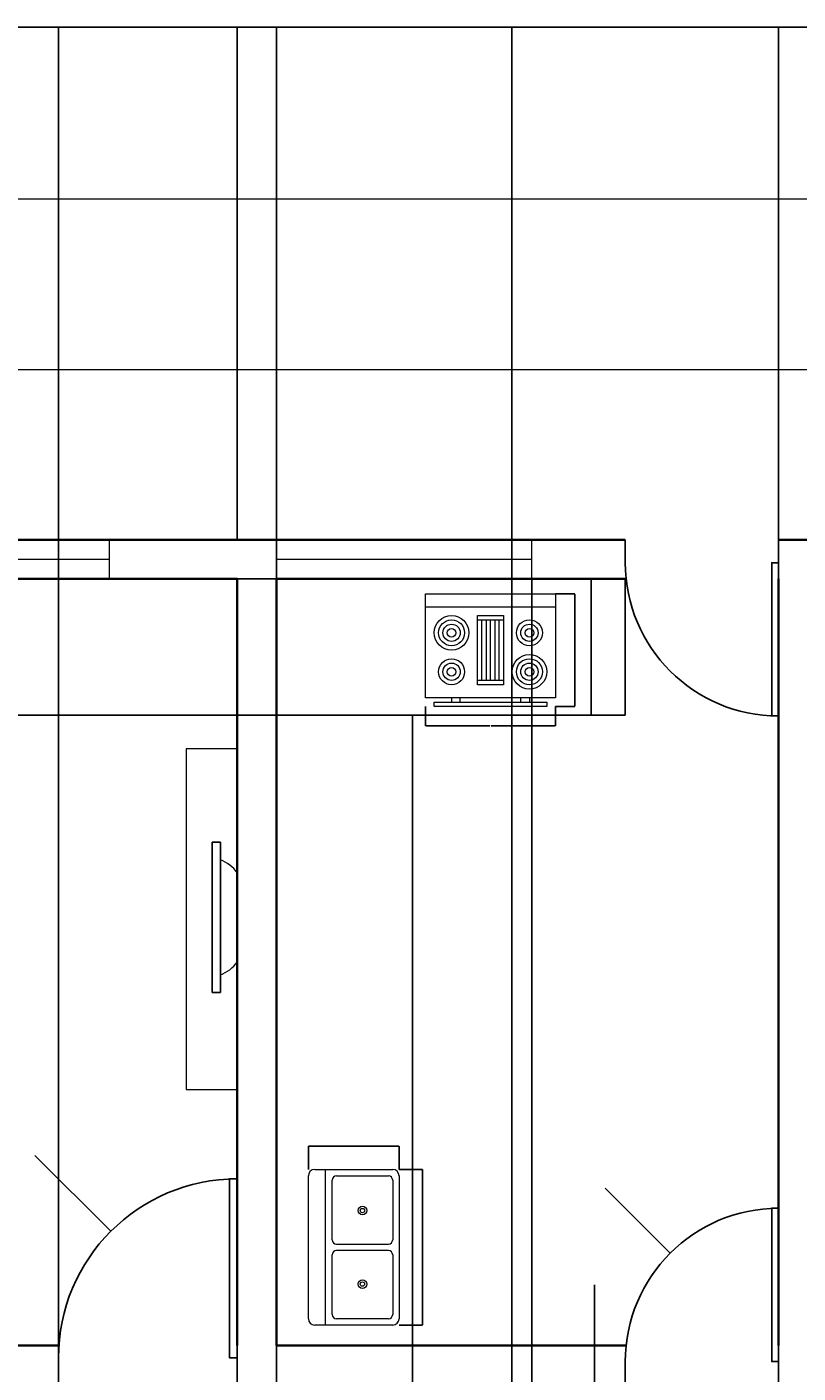
# Model space of a CAD drawing. Units: millimetres. Extents: x -8052 to 19968, y -37825 to -17505.
# Tile 7 of 10: x -516 to 4015, y -25407 to -17505. Entities that reach past the tile are written whole.
import ezdxf

# ---------------------------------------------------------------- set-up
doc = ezdxf.new("R2010")
doc.units = ezdxf.units.MM
doc.header["$MEASUREMENT"] = 0
for name, color, linetype, lineweight in [('A-ANNO-DIMS', 2, 'Continuous', 18), ('A-DOOR', 3, 'Continuous', 25), ('A-EQPM', 8, 'Continuous', 18), ('A-FLOR', 8, 'Continuous', 18), ('A-FLOR-CASE', 9, 'Continuous', 25), ('A-FLOR-FIXT', 9, 'Continuous', 18), ('A-GLAZ', 4, 'Continuous', 18), ('A-WALL', 7, 'Continuous', 35)]:
    doc.layers.add(name, color=color, linetype=linetype, lineweight=lineweight)
doc.styles.get("Standard").update_dxf_attribs({"font": 'arial.ttf'})
doc.dimstyles.get("Standard").update_dxf_attribs({"dimtxt": 1.054, "dimasz": 1.055, "dimexe": 0.18, "dimexo": 0.0625, "dimgap": 0.09, "dimtad": 0, "dimtih": 1, "dimtoh": 1, "dimdec": 4, "dimzin": 0, "dimdsep": 46, "dimtxsty": 'Standard', "dimcen": 0.09, "dimadec": 0, "dimazin": 0, "dimtfac": 1, "dimtdec": 4, "dimtofl": 0, "dimtmove": 0, "dimatfit": 3, "dimfxl": 1, "dimtolj": 1, "dimtzin": 0, "dimarcsym": 0})

# ---------------------------------------------------------------- blocks, each defined once
blk = doc.blocks.new('*U10')
for p, q in [((0, 0), (0, -6)), ((40, 0), (40, -6))]:
    blk.add_line(p, q)
blk.add_lwpolyline([(0, 0), (0, 40), (1.75, 40), (1.75, 0)], close=True)
blk.add_arc((0, 0), 40, 0, 90)
blk = doc.blocks.new('Range-Oven - 30 in top')
for p, q in [((0, -3), (30, -3)), ((12, -6), (18, -6)), ((13, -20), (13, -6)), ((14, -6), (14, -20)), ((15, -20), (15, -6)), ((16, -6), (16, -20)), ((17, -20), (17, -6)), ((18, -20), (12, -20)), ((6, -24), (6, -25)), ((8, -25), (8, -24)), ((22, -25), (22, -24)), ((24, -24), (24, -25))]:
    blk.add_line(p, q)
for points in [[(0, -24), (0, 0), (30, 0), (30, -24)], [(12, -21), (12, -5), (18, -5), (18, -21)], [(2, -26), (2, -25), (28, -25), (28, -26)]]:
    blk.add_lwpolyline(points, close=True)
for centre, radius in [((6, -9), 4), ((6, -9), 3), ((24, -9), 3), ((6, -9), 2), ((6, -9), 1), ((24, -9), 2), ((24, -9), 1), ((6, -18), 3), ((24, -18), 4), ((24, -18), 3), ((6, -18), 2), ((6, -18), 1), ((24, -18), 2), ((24, -18), 1)]:
    blk.add_circle(centre, radius)
blk = doc.blocks.new('Sink-double - 36 in top')
for p, q in [((-18, -4), (18, -4)), ((-0.75, -18.5), (-0.75, -6.5)), ((0.75, -6.5), (0.75, -18.5))]:
    blk.add_line(p, q)
for points in [[(-16.5, 0), (16.5, 0)], [(-18, -19.5), (-18, -1.5)], [(18, -1.5), (18, -19.5)], [(-15.5, -5.5), (-1.75, -5.5)], [(1.75, -5.5), (15.5, -5.5)], [(-16.5, -18.5), (-16.5, -6.5)], [(16.5, -6.5), (16.5, -18.5)], [(16.5, -21), (-16.5, -21)], [(-1.75, -19.5), (-15.5, -19.5)], [(15.5, -19.5), (1.75, -19.5)]]:
    blk.add_lwpolyline(points)
for centre, radius in [((-8.5, -12.5), 1), ((-8.5, -12.5), 0.5), ((8.5, -12.5), 1), ((8.5, -12.5), 0.5)]:
    blk.add_circle(centre, radius)
for centre, radius, start, end in [((-16.5, -1.5), 1.5, 90, 180), ((16.5, -1.5), 1.5, 0, 90), ((-15.5, -6.5), 1, 90, 180), ((-1.75, -6.5), 1, 0, 90), ((1.75, -6.5), 1, 90, 180), ((15.5, -6.5), 1, 0, 90), ((-15.5, -18.5), 1, 180, 270), ((-1.75, -18.5), 1, 270, 0), ((1.75, -18.5), 1, 180, 270), ((15.5, -18.5), 1, 270, 0), ((-16.5, -19.5), 1.5, 180, 270), ((16.5, -19.5), 1.5, 270, 0)]:
    blk.add_arc(centre, radius, start, end)
blk = doc.blocks.new('MEDIA-CONSOLE-2000')
for points in [[(300, 2000), (0, 2000), (0, 0), (300, 0)], [(201.6, 1452.1), (152.5, 1452.1), (152.5, 569.2), (201.6, 569.2)], [(201.6, 569.2), (152.5, 569.2), (152.5, 1452.1), (201.6, 1452.1)]]:
    blk.add_lwpolyline(points, close=True)
for centre, start, end in [((115.1, 1133.4), 37.07446, 68.10078), ((115.1, 887.8), 291.89922, 322.92554)]:
    blk.add_arc(centre, 231.7, start, end)
blk = doc.blocks.new('WIN-2000')
for p, q in [((0, 0), (0, 230)), ((2000, 0), (2000, 230)), ((0, 115), (2000, 115))]:
    blk.add_line(p, q)
blk = doc.blocks.new('*D76')
at = {"layer": 'A-ANNO-DIMS', "color": 0, "lineweight": -2, "transparency": 16777216}
for p, q in [((1827, -21493.5), (1827, -21607.9)), ((2589, -21493.5), (2589, -21607.9)), ((1828.1, -21607.7), (2204, -21607.7)), ((2588, -21607.7), (2212.1, -21607.7))]:
    blk.add_line(p, q, dxfattribs=at)
at = {"layer": 'A-ANNO-DIMS', "color": 0, "lineweight": 100, "transparency": 16777216}
for points in [[(1828.1, -21607.5), (1828.1, -21607.9), (1827, -21607.7)], [(2588, -21607.5), (2588, -21607.9), (2589, -21607.7)]]:
    blk.add_solid(points, dxfattribs=at)
at = {"layer": 'Defpoints', "color": 0, "lineweight": 100, "transparency": 16777216}
for p in [(1827, -21493.4), (2589, -21493.4), (2589, -21607.7)]:
    blk.add_point(p, dxfattribs=at)
at = {"layer": 'A-ANNO-DIMS', "color": 0, "transparency": 16777216, "insert": (2208, -21607.7), "char_height": 1.054, "attachment_point": 5}
blk.add_mtext('\\A1;RANGE 762', dxfattribs=at)
blk = doc.blocks.new('*D77')
at = {"layer": 'A-ANNO-DIMS', "color": 0, "lineweight": -2, "transparency": 16777216}
for p, q in [((2589.1, -20833), (2703.5, -20833)), ((2703.3, -20834.1), (2703.3, -21162.6)), ((2703.3, -21492.3), (2703.3, -21163.8)), ((2589.1, -21493.4), (2703.5, -21493.4))]:
    blk.add_line(p, q, dxfattribs=at)
at = {"layer": 'A-ANNO-DIMS', "color": 0, "lineweight": 100, "transparency": 16777216}
for points in [[(2703.2, -20834.1), (2703.5, -20834.1), (2703.3, -20833)], [(2703.2, -21492.3), (2703.5, -21492.3), (2703.3, -21493.4)]]:
    blk.add_solid(points, dxfattribs=at)
at = {"layer": 'Defpoints', "color": 0, "lineweight": 100, "transparency": 16777216}
for p in [(2589, -20833), (2703.3, -20833), (2589, -21493.4)]:
    blk.add_point(p, dxfattribs=at)
at = {"layer": 'A-ANNO-DIMS', "color": 0, "transparency": 16777216, "insert": (2703.3, -21163.2), "char_height": 1.05, "attachment_point": 5}
blk.add_mtext('\\A1;660', dxfattribs=at)
blk = doc.blocks.new('*D78')
at = {"layer": 'A-ANNO-DIMS', "color": 0, "lineweight": -2, "transparency": 16777216}
for p, q in [((1671.4, -24211.8), (1808.7, -24211.8)), ((1808.5, -24212.8), (1808.5, -24668.3)), ((1808.5, -25125.1), (1808.5, -24669.6)), ((1671.4, -25126.2), (1808.7, -25126.2))]:
    blk.add_line(p, q, dxfattribs=at)
at = {"layer": 'A-ANNO-DIMS', "color": 0, "lineweight": 100, "transparency": 16777216}
for points in [[(1808.3, -24212.8), (1808.7, -24212.8), (1808.5, -24211.8)], [(1808.3, -25125.1), (1808.7, -25125.1), (1808.5, -25126.2)]]:
    blk.add_solid(points, dxfattribs=at)
at = {"layer": 'Defpoints', "color": 0, "lineweight": 100, "transparency": 16777216}
for p in [(1671.4, -24211.8), (1808.5, -24211.8), (1671.4, -25126.2)]:
    blk.add_point(p, dxfattribs=at)
at = {"layer": 'A-ANNO-DIMS', "color": 0, "transparency": 16777216, "insert": (1808.5, -24669), "char_height": 1.054, "attachment_point": 5}
blk.add_mtext('\\A1;DOUBLE SINK 914', dxfattribs=at)
blk = doc.blocks.new('*D79')
at = {"layer": 'A-ANNO-DIMS', "color": 0, "lineweight": -2, "transparency": 16777216}
for p, q in [((1138, -24211.7), (1138, -24074.4)), ((1139, -24074.6), (1403.4, -24074.6)), ((1670.3, -24074.6), (1405.9, -24074.6)), ((1671.4, -24211.7), (1671.4, -24074.4))]:
    blk.add_line(p, q, dxfattribs=at)
at = {"layer": 'A-ANNO-DIMS', "color": 0, "lineweight": 100, "transparency": 16777216}
for points in [[(1139, -24074.4), (1139, -24074.8), (1138, -24074.6)], [(1670.3, -24074.4), (1670.3, -24074.8), (1671.4, -24074.6)]]:
    blk.add_solid(points, dxfattribs=at)
at = {"layer": 'Defpoints', "color": 0, "lineweight": 100, "transparency": 16777216}
for p in [(1138, -24074.6), (1138, -24211.8), (1671.4, -24211.8)]:
    blk.add_point(p, dxfattribs=at)
at = {"layer": 'A-ANNO-DIMS', "color": 0, "transparency": 16777216, "insert": (1404.7, -24074.6), "char_height": 1.05, "attachment_point": 5}
blk.add_mtext('\\A1;533', dxfattribs=at)
blk = doc.blocks.new('*D84')
at = {"layer": 'A-ANNO-DIMS', "color": 0, "lineweight": -2, "transparency": 16777216}
for p, q in [((-7040, -18514.8), (-7040, -17505.2)), ((-7039, -17505.3), (3022.9, -17505.3)), ((13088.9, -17505.3), (3027.1, -17505.3)), ((13090, -18514.8), (13090, -17505.2))]:
    blk.add_line(p, q, dxfattribs=at)
at = {"layer": 'A-ANNO-DIMS', "color": 0, "lineweight": 100, "transparency": 16777216}
for points in [[(-7039, -17505.2), (-7039, -17505.5), (-7040, -17505.3)], [(13088.9, -17505.2), (13088.9, -17505.5), (13090, -17505.3)]]:
    blk.add_solid(points, dxfattribs=at)
at = {"layer": 'Defpoints', "color": 0, "lineweight": 100, "transparency": 16777216}
for p in [(13090, -17505.3), (-7040, -18514.8), (13090, -18514.8)]:
    blk.add_point(p, dxfattribs=at)
at = {"layer": 'A-ANNO-DIMS', "color": 0, "transparency": 16777216, "insert": (3025, -17505.3), "char_height": 1.05, "attachment_point": 5}
blk.add_mtext('\\A1;20130', dxfattribs=at)
blk = doc.blocks.new('*D90')
at = {"layer": 'A-ANNO-DIMS', "color": 0, "lineweight": -2, "transparency": 16777216}
for p, q in [((-3010, -20514.8), (-3010, -17505.2)), ((-3009, -17505.3), (-1146.7, -17505.3)), ((718.9, -17505.3), (-1143.4, -17505.3)), ((720, -20514.8), (720, -17505.2))]:
    blk.add_line(p, q, dxfattribs=at)
at = {"layer": 'A-ANNO-DIMS', "color": 0, "lineweight": 100, "transparency": 16777216}
for points in [[(-3009, -17505.2), (-3009, -17505.5), (-3010, -17505.3)], [(718.9, -17505.2), (718.9, -17505.5), (720, -17505.3)]]:
    blk.add_solid(points, dxfattribs=at)
at = {"layer": 'Defpoints', "color": 0, "lineweight": 100, "transparency": 16777216}
for p in [(720, -17505.3), (-3010, -20514.8), (720, -20514.8)]:
    blk.add_point(p, dxfattribs=at)
at = {"layer": 'A-ANNO-DIMS', "color": 0, "transparency": 16777216, "insert": (-1145, -17505.3), "char_height": 1.05, "attachment_point": 5}
blk.add_mtext('\\A1;3730', dxfattribs=at)
blk = doc.blocks.new('*D91')
at = {"layer": 'A-ANNO-DIMS', "color": 0, "lineweight": -2, "transparency": 16777216}
for p, q in [((720, -20514.8), (720, -17505.2)), ((721, -17505.3), (2308.3, -17505.3)), ((3898.9, -17505.3), (2311.6, -17505.3)), ((3900, -20514.8), (3900, -17505.2))]:
    blk.add_line(p, q, dxfattribs=at)
at = {"layer": 'A-ANNO-DIMS', "color": 0, "lineweight": 100, "transparency": 16777216}
for points in [[(721, -17505.2), (721, -17505.5), (720, -17505.3)], [(3898.9, -17505.2), (3898.9, -17505.5), (3900, -17505.3)]]:
    blk.add_solid(points, dxfattribs=at)
at = {"layer": 'Defpoints', "color": 0, "lineweight": 100, "transparency": 16777216}
for p in [(3900, -17505.3), (720, -20514.8), (3900, -20514.8)]:
    blk.add_point(p, dxfattribs=at)
at = {"layer": 'A-ANNO-DIMS', "color": 0, "transparency": 16777216, "insert": (2310, -17505.3), "char_height": 1.05, "attachment_point": 5}
blk.add_mtext('\\A1;3180', dxfattribs=at)
blk = doc.blocks.new('*D92')
at = {"layer": 'A-ANNO-DIMS', "color": 0, "lineweight": -2, "transparency": 16777216}
for p, q in [((3900, -20514.8), (3900, -17505.2)), ((3901, -17505.3), (6513.3, -17505.3)), ((9128.9, -17505.3), (6516.6, -17505.3)), ((9130, -20514.8), (9130, -17505.2))]:
    blk.add_line(p, q, dxfattribs=at)
at = {"layer": 'A-ANNO-DIMS', "color": 0, "lineweight": 100, "transparency": 16777216}
for points in [[(3901, -17505.2), (3901, -17505.5), (3900, -17505.3)], [(9128.9, -17505.2), (9128.9, -17505.5), (9130, -17505.3)]]:
    blk.add_solid(points, dxfattribs=at)
at = {"layer": 'Defpoints', "color": 0, "lineweight": 100, "transparency": 16777216}
for p in [(9130, -17505.3), (3900, -20514.8), (9130, -20514.8)]:
    blk.add_point(p, dxfattribs=at)
at = {"layer": 'A-ANNO-DIMS', "color": 0, "transparency": 16777216, "insert": (6515, -17505.3), "char_height": 1.05, "attachment_point": 5}
blk.add_mtext('\\A1;5230', dxfattribs=at)
blk = doc.blocks.new('*D108')
at = {"layer": 'A-ANNO-DIMS', "color": 0, "lineweight": -2, "transparency": 16777216}
for p, q in [((-330, -29974.8), (-330, -17505.2)), ((-329, -17505.3), (3348.3, -17505.3)), ((7028.9, -17505.3), (3351.6, -17505.3)), ((7030, -29974.8), (7030, -17505.2))]:
    blk.add_line(p, q, dxfattribs=at)
at = {"layer": 'A-ANNO-DIMS', "color": 0, "lineweight": 100, "transparency": 16777216}
for points in [[(-329, -17505.2), (-329, -17505.5), (-330, -17505.3)], [(7028.9, -17505.2), (7028.9, -17505.5), (7030, -17505.3)]]:
    blk.add_solid(points, dxfattribs=at)
at = {"layer": 'Defpoints', "color": 0, "lineweight": 100, "transparency": 16777216}
for p in [(7030, -17505.3), (-330, -29974.8), (7030, -29974.8)]:
    blk.add_point(p, dxfattribs=at)
at = {"layer": 'A-ANNO-DIMS', "color": 0, "transparency": 16777216, "insert": (3350, -17505.3), "char_height": 1.05, "attachment_point": 5}
blk.add_mtext('\\A1;7360', dxfattribs=at)
blk = doc.blocks.new('*D113')
at = {"layer": 'A-ANNO-DIMS', "color": 0, "lineweight": -2, "transparency": 16777216}
for p, q in [((950, -25244.9), (950, -37824.5)), ((1750, -25244.9), (1750, -37824.5)), ((951, -37824.3), (1348.7, -37824.3)), ((1748.9, -37824.3), (1351.2, -37824.3))]:
    blk.add_line(p, q, dxfattribs=at)
at = {"layer": 'A-ANNO-DIMS', "color": 0, "lineweight": 100, "transparency": 16777216}
for points in [[(951, -37824.2), (951, -37824.5), (950, -37824.3)], [(1748.9, -37824.2), (1748.9, -37824.5), (1750, -37824.3)]]:
    blk.add_solid(points, dxfattribs=at)
at = {"layer": 'Defpoints', "color": 0, "lineweight": 100, "transparency": 16777216}
for p in [(950, -25244.8), (1750, -25244.8), (1750, -37824.3)]:
    blk.add_point(p, dxfattribs=at)
at = {"layer": 'A-ANNO-DIMS', "color": 0, "transparency": 16777216, "insert": (1350, -37824.3), "char_height": 1.05, "attachment_point": 5}
blk.add_mtext('\\A1;800', dxfattribs=at)
blk = doc.blocks.new('*D114')
at = {"layer": 'A-ANNO-DIMS', "color": 0, "lineweight": -2, "transparency": 16777216}
for p, q in [((2999.9, -20744.8), (-8049.7, -20744.8)), ((-8049.5, -20745.9), (-8049.5, -21144.2)), ((-8049.5, -21543.8), (-8049.5, -21145.5)), ((2999.9, -21544.8), (-8049.7, -21544.8))]:
    blk.add_line(p, q, dxfattribs=at)
at = {"layer": 'A-ANNO-DIMS', "color": 0, "lineweight": 100, "transparency": 16777216}
for points in [[(-8049.7, -20745.9), (-8049.3, -20745.9), (-8049.5, -20744.8)], [(-8049.7, -21543.8), (-8049.3, -21543.8), (-8049.5, -21544.8)]]:
    blk.add_solid(points, dxfattribs=at)
at = {"layer": 'Defpoints', "color": 0, "lineweight": 100, "transparency": 16777216}
for p in [(3000, -20744.8), (-8049.5, -21544.8), (3000, -21544.8)]:
    blk.add_point(p, dxfattribs=at)
at = {"layer": 'A-ANNO-DIMS', "color": 0, "transparency": 16777216, "insert": (-8049.5, -21144.8), "char_height": 1.05, "attachment_point": 5}
blk.add_mtext('\\A1;800', dxfattribs=at)
blk = doc.blocks.new('*D115')
at = {"layer": 'A-ANNO-DIMS', "color": 0, "lineweight": -2, "transparency": 16777216}
for p, q in [((950, -20744.9), (950, -37824.5)), ((2450, -20744.9), (2450, -37824.5)), ((951, -37824.3), (1698.4, -37824.3)), ((2448.9, -37824.3), (1701.6, -37824.3))]:
    blk.add_line(p, q, dxfattribs=at)
at = {"layer": 'A-ANNO-DIMS', "color": 0, "lineweight": 100, "transparency": 16777216}
for points in [[(951, -37824.2), (951, -37824.5), (950, -37824.3)], [(2448.9, -37824.2), (2448.9, -37824.5), (2450, -37824.3)]]:
    blk.add_solid(points, dxfattribs=at)
at = {"layer": 'Defpoints', "color": 0, "lineweight": 100, "transparency": 16777216}
for p in [(950, -20744.8), (2450, -20744.8), (2450, -37824.3)]:
    blk.add_point(p, dxfattribs=at)
at = {"layer": 'A-ANNO-DIMS', "color": 0, "transparency": 16777216, "insert": (1700, -37824.3), "char_height": 1.05, "attachment_point": 5}
blk.add_mtext('\\A1;1500', dxfattribs=at)
blk = doc.blocks.new('*D118')
at = {"layer": 'A-ANNO-DIMS', "color": 0, "lineweight": -2, "transparency": 16777216}
for p, q in [((950, -33624.8), (950, -17505.2)), ((951, -17505.3), (1640.4, -17505.3)), ((2332.9, -17505.3), (1643.6, -17505.3)), ((2334, -33624.8), (2334, -17505.2))]:
    blk.add_line(p, q, dxfattribs=at)
at = {"layer": 'A-ANNO-DIMS', "color": 0, "lineweight": 100, "transparency": 16777216}
for points in [[(951, -17505.2), (951, -17505.5), (950, -17505.3)], [(2332.9, -17505.2), (2332.9, -17505.5), (2334, -17505.3)]]:
    blk.add_solid(points, dxfattribs=at)
at = {"layer": 'Defpoints', "color": 0, "lineweight": 100, "transparency": 16777216}
for p in [(2334, -17505.3), (950, -33624.8), (2334, -33624.8)]:
    blk.add_point(p, dxfattribs=at)
at = {"layer": 'A-ANNO-DIMS', "color": 0, "transparency": 16777216, "insert": (1642, -17505.3), "char_height": 1.05, "attachment_point": 5}
blk.add_mtext('\\A1;1384', dxfattribs=at)
blk = doc.blocks.new('*D131')
at = {"layer": 'A-ANNO-DIMS', "color": 0, "lineweight": -2, "transparency": 16777216}
for p, q in [((-469, -24129.4), (-468, -24129.4)), ((-468, -24129.4), (-23.2, -24574.1)), ((719.9, -25317.3), (720.1, -25317.3)), ((720, -25317.4), (720, -25317.3))]:
    blk.add_line(p, q, dxfattribs=at)
at = {"layer": 'A-ANNO-DIMS', "color": 0, "lineweight": 100, "transparency": 16777216}
blk.add_solid([(-23.1, -24574), (-23.4, -24574.3), (-22.5, -24574.9)], dxfattribs=at)
at = {"layer": 'Defpoints', "color": 0, "lineweight": 100, "transparency": 16777216}
for p in [(-22.5, -24574.9), (720, -25317.3)]:
    blk.add_point(p, dxfattribs=at)
at = {"layer": 'A-ANNO-DIMS', "color": 0, "transparency": 16777216, "insert": (-471.2, -24129.4), "char_height": 1.05, "attachment_point": 5}
blk.add_mtext('\\A1;R1050', dxfattribs=at)
blk = doc.blocks.new('*D132')
at = {"layer": 'A-ANNO-DIMS', "color": 0, "lineweight": -2, "transparency": 16777216}
for p, q in [((2880.7, -24321.6), (2881.7, -24321.6)), ((2881.7, -24321.6), (3262.8, -24702.7)), ((3899.9, -25339.8), (3900.1, -25339.8)), ((3900, -25339.9), (3900, -25339.8))]:
    blk.add_line(p, q, dxfattribs=at)
at = {"layer": 'A-ANNO-DIMS', "color": 0, "lineweight": 100, "transparency": 16777216}
blk.add_solid([(3263, -24702.6), (3262.7, -24702.8), (3263.6, -24703.5)], dxfattribs=at)
at = {"layer": 'Defpoints', "color": 0, "lineweight": 100, "transparency": 16777216}
for p in [(3263.6, -24703.5), (3900, -25339.8)]:
    blk.add_point(p, dxfattribs=at)
at = {"layer": 'A-ANNO-DIMS', "color": 0, "transparency": 16777216, "insert": (2878.9, -24321.6), "char_height": 1.05, "attachment_point": 5}
blk.add_mtext('\\A1;R900', dxfattribs=at)
blk = doc.blocks.new('*D135')
at = {"layer": 'A-ANNO-DIMS', "color": 0, "lineweight": -2, "transparency": 16777216}
for p, q in [((2819.8, -24888.5), (2818.7, -24888.5)), ((2818.7, -24888.5), (2818.7, -25805.6)), ((2818.7, -27337), (2818.8, -27337)), ((2818.7, -27337.1), (2818.7, -27337))]:
    blk.add_line(p, q, dxfattribs=at)
at = {"layer": 'A-ANNO-DIMS', "color": 0, "lineweight": 100, "transparency": 16777216}
blk.add_solid([(2818.6, -25805.6), (2818.9, -25805.6), (2818.7, -25806.7)], dxfattribs=at)
at = {"layer": 'Defpoints', "color": 0, "lineweight": 100, "transparency": 16777216}
for p in [(2818.7, -25806.7), (2818.7, -27337)]:
    blk.add_point(p, dxfattribs=at)
at = {"layer": 'A-ANNO-DIMS', "color": 0, "transparency": 16777216, "insert": (2823.7, -24888.5), "char_height": 1.054, "attachment_point": 5}
blk.add_mtext('\\A1;2X R1530.3', dxfattribs=at)

msp = doc.modelspace()

# ---------------------------------------------------------------- linework, layer by layer
at = {"layer": 'A-DOOR'}
for p, q in [((-330.021, -25317.343), (-330.021, -25474.843)), ((719.979, -25317.343), (719.979, -25474.843)), ((2999.979, -25339.843), (2999.979, -25474.843)), ((3899.979, -25339.843), (3899.979, -25474.843))]:
    msp.add_line(p, q, dxfattribs=at)
for points in [[(719.979, -25317.343), (719.979, -24267.343), (674.042, -24267.343), (674.042, -25317.343)], [(3899.979, -25339.843), (3899.979, -24439.843), (3860.604, -24439.843), (3860.604, -25339.843)]]:
    msp.add_lwpolyline(points, close=True, dxfattribs=at)
for centre, radius in [((719.979, -25317.343), 1050), ((3899.979, -25339.843), 900)]:
    msp.add_arc(centre, radius, 90, 180, dxfattribs=at)
at = {"layer": 'A-FLOR'}
for p, q in [((-4810.021, -18514.843), (13089.979, -18514.843)), ((-6040.021, -19514.843), (12089.979, -19514.843))]:
    msp.add_line(p, q, dxfattribs=at)
at = {"layer": 'A-FLOR-CASE'}
for p, q in [((2799.979, -20744.843), (2799.979, -21244.843)), ((2999.979, -20744.843), (2999.979, -21244.843)), ((2799.979, -21244.843), (2799.979, -21344.843)), ((2999.979, -21244.843), (2999.979, -21344.843)), ((2799.979, -21344.843), (2799.979, -21544.843)), ((2999.979, -21344.843), (2999.979, -21544.843)), ((1749.979, -21544.843), (1749.979, -25244.843)), ((2799.979, -21544.843), (1749.979, -21544.843)), ((2999.979, -21544.843), (2799.979, -21544.843))]:
    msp.add_line(p, q, dxfattribs=at)
at = {"layer": 'A-GLAZ'}
for p, q in [((949.979, -20744.843), (949.979, -20514.843)), ((2449.979, -20744.843), (2449.979, -20514.843)), ((949.979, -20629.843), (2449.979, -20629.843))]:
    msp.add_line(p, q, dxfattribs=at)
at = {"layer": 'A-WALL'}
for p, q in [((-2780.021, -20514.843), (719.979, -20514.843)), ((719.979, -20514.843), (949.979, -20514.843)), ((949.979, -20514.843), (2999.979, -20514.843)), ((3899.979, -20514.843), (4129.979, -20514.843)), ((-2780.021, -20744.843), (719.979, -20744.843)), ((719.979, -25244.843), (719.979, -20744.843)), ((949.979, -20744.843), (949.979, -25244.843)), ((949.979, -20744.843), (2999.979, -20744.843)), ((3899.979, -25244.843), (3899.979, -20744.843)), ((-2780.021, -25244.843), (-330.021, -25244.843)), ((949.979, -25244.843), (3005.033, -25244.6))]:
    msp.add_line(p, q, dxfattribs=at)

# ---------------------------------------------------------------- block references
at = {"layer": 'A-DOOR', "xscale": 22.5, "yscale": 22.5, "zscale": 22.5, "rotation": 180}
msp.add_blockref('*U10', (3899.979, -20649.843), dxfattribs=at)
at = {"layer": 'A-EQPM', "xscale": 25.4, "yscale": 25.4, "zscale": 25.4}
msp.add_blockref('Range-Oven - 30 in top', (1827.034, -20833.003), dxfattribs=at)
at = {"layer": 'A-EQPM'}
msp.add_blockref('MEDIA-CONSOLE-2000', (419.979, -23742.93), dxfattribs=at)
at = {"layer": 'A-FLOR-FIXT', "xscale": 25.4, "yscale": 25.4, "zscale": 25.4, "rotation": 90}
msp.add_blockref('Sink-double - 36 in top', (1137.959, -24668.965), dxfattribs=at)
at = {"layer": 'A-GLAZ'}
msp.add_blockref('WIN-2000', (-2030.021, -20744.843), dxfattribs=at)

# ---------------------------------------------------------------- dimensions: what is measured, and where the dimension line sits
at = {"layer": 'A-ANNO-DIMS'}
for base, p1, p2, picture, middle in [((13089.979, -17505.343), (-7040.021, -18514.843), (13089.979, -18514.843), '*D84', (3024.979, -17505.343)), ((719.979, -17505.343), (-3010.021, -20514.843), (719.979, -20514.843), '*D90', (-1145.021, -17505.343)), ((7029.979, -17505.343), (-330.021, -29974.843), (7029.979, -29974.843), '*D108', (3349.979, -17505.343)), ((3899.979, -17505.343), (719.979, -20514.843), (3899.979, -20514.843), '*D91', (2309.979, -17505.343)), ((2333.979, -17505.343), (949.979, -33624.843), (2333.979, -33624.843), '*D118', (1641.979, -17505.343)), ((9129.979, -17505.343), (3899.979, -20514.843), (9129.979, -20514.843), '*D92', (6514.979, -17505.343)), ((2449.979, -37824.343), (949.979, -20744.843), (2449.979, -20744.843), '*D115', (1699.979, -37824.343)), ((1749.979, -37824.343), (949.979, -25244.843), (1749.979, -25244.843), '*D113', (1349.979, -37824.343))]:
    dim = msp.add_linear_dim(base=base, p1=p1, p2=p2, dimstyle='Standard', override={"dimdec": 0, "dimlfac": 1, "dimrnd": 0, "dimzin": 0, "dimdsep": 46, "dimlunit": 2}, dxfattribs=at)
    dim.commit()
    dim.dimension.update_dxf_attribs({"geometry": picture, "text_midpoint": middle})
for base, p1, p2, angle, picture, middle in [((-8049.521, -21544.843), (2999.979, -20744.843), (2999.979, -21544.843), 90, '*D114', (-8049.521, -21144.843)), ((2703.334, -20833.003), (2589.034, -21493.403), (2589.034, -20833.003), 90, '*D77', (2703.334, -21163.203)), ((1137.959, -24074.605), (1671.359, -24211.765), (1137.959, -24211.765), 180, '*D79', (1404.659, -24074.605))]:
    dim = msp.add_linear_dim(base=base, p1=p1, p2=p2, angle=angle, dimstyle='Standard', override={"dimdec": 0, "dimlfac": 1, "dimrnd": 0, "dimzin": 0, "dimdsep": 46, "dimlunit": 2}, dxfattribs=at)
    dim.commit()
    dim.dimension.update_dxf_attribs({"geometry": picture, "text_midpoint": middle})
dim = msp.add_linear_dim(base=(2589.034, -21607.703), p1=(1827.034, -21493.403), p2=(2589.034, -21493.403), text='RANGE <>', dimstyle='Standard', override={"dimdec": 0, "dimlfac": 1, "dimrnd": 0, "dimzin": 0, "dimdsep": 46, "dimlunit": 2}, dxfattribs=at)
dim.commit()
dim.dimension.update_dxf_attribs({"geometry": '*D76', "text_midpoint": (2208.034, -21607.703)})
for center, mpoint, picture, middle in [((719.979, -25317.343), (-22.481, -24574.879), '*D131', (-471.178, -24129.401)), ((3899.979, -25339.843), (3263.58, -24703.45), '*D132', (2878.929, -24321.614))]:
    dim = msp.add_radius_dim(center=center, mpoint=mpoint, dimstyle='Standard', override={"dimdec": 0, "dimlfac": 1, "dimrnd": 0, "dimzin": 0, "dimdsep": 46, "dimlunit": 2}, dxfattribs=at)
    dim.commit()
    dim.dimension.update_dxf_attribs({"geometry": picture, "text_midpoint": middle, "dimtype": 164})
dim = msp.add_linear_dim(base=(1808.519, -24211.765), p1=(1671.359, -25126.165), p2=(1671.359, -24211.765), angle=90, text='DOUBLE SINK <>', dimstyle='Standard', override={"dimdec": 0, "dimlfac": 1, "dimrnd": 0, "dimzin": 0, "dimdsep": 46, "dimlunit": 2}, dxfattribs=at)
dim.commit()
dim.dimension.update_dxf_attribs({"geometry": '*D78', "text_midpoint": (1808.519, -24668.965)})
dim = msp.add_radius_dim(center=(2818.747, -27337.042), mpoint=(2818.747, -25806.693), text='2X <>', dimstyle='Standard', override={"dimdec": 1, "dimlfac": 1, "dimrnd": 0, "dimzin": 0, "dimdsep": 46, "dimlunit": 2}, dxfattribs=at)
dim.commit()
dim.dimension.update_dxf_attribs({"geometry": '*D135', "text_midpoint": (2823.726, -24888.483), "dimtype": 164})

doc.saveas('drawing.dxf')
